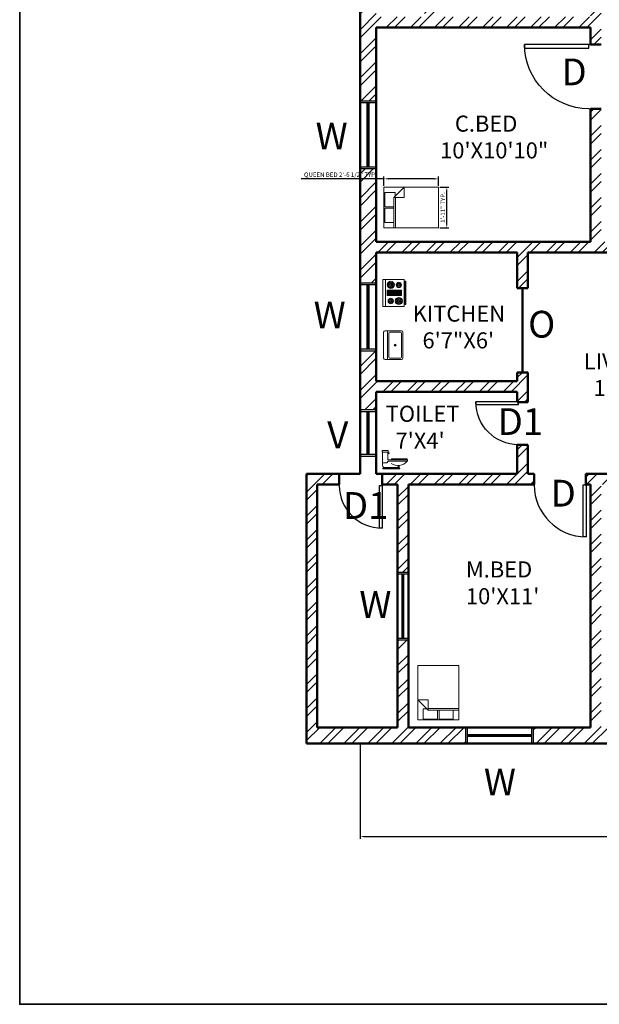
# Model space of a CAD drawing. Units: inches. Extents: x -31842 to -29388, y 18869 to 19743.
# Tile 1 of 12: x -31842 to -31517, y 18869 to 19420. Entities that reach past the tile are written whole.
import ezdxf

# ---------------------------------------------------------------- set-up
doc = ezdxf.new("R2010")
doc.units = ezdxf.units.IN
for name, color, linetype, lineweight in [('A-ANNO-DIMS', 2, 'Continuous', 18), ('A-ANNO-SYMB', 2, 'Continuous', 18), ('A-ANNO-TTLB', 7, 'Continuous', 35), ('A-AREA-IDEN', 3, 'Continuous', 18), ('A-DOOR', 3, 'Continuous', 25), ('A-FLOR-FIXT', 8, 'Continuous', 18), ('A-FURN', 8, 'Continuous', 18), ('A-GLAZ', 4, 'Continuous', 25), ('A-WALL', 7, 'Continuous', 50), ('A-WALL-PATT', 8, 'Continuous', 13)]:
    doc.layers.add(name, color=color, linetype=linetype, lineweight=lineweight)
doc.styles.get("Standard").update_dxf_attribs({"font": 'arial.ttf'})
doc.dimstyles.new('ISO-25', dxfattribs={"dimtxt": 2.5, "dimasz": 2.5, "dimexe": 1.25, "dimexo": 0.625, "dimtad": 1, "dimdec": 0, "dimlunit": 3, "dimtxsty": 'Standard', "dimcen": 2.5, "dimadec": 0, "dimazin": 0, "dimtfac": 1, "dimtdec": 0, "dimtmove": 0, "dimatfit": 3, "dimfxl": 1, "dimarcsym": 0})

# ---------------------------------------------------------------- blocks, each defined once
blk = doc.blocks.new('*U8')
for p, q in [((0, 0), (0, -100)), ((750, 0), (750, -100))]:
    blk.add_line(p, q)
blk.add_lwpolyline([(0, 0), (0, 750), (43.75, 750), (43.75, 0)], close=True)
blk.add_arc((0, 0), 750, 0, 90)
blk = doc.blocks.new('Bed - Queen')
for p, q in [((0, -80.00003), (0, 0)), ((0, 0), (59.99999, 0)), ((59.99999, 0), (59.99999, -80.00003)), ((0, -14.4), (44.8, -14.4)), ((7.99999, -1.2), (28.79998, -1.2)), ((7.99999, -14.4), (7.99999, -1.2)), ((28.79998, -1.2), (28.79998, -14.4)), ((31.19999, -1.2), (51.99999, -1.2)), ((31.19999, -14.4), (31.19999, -1.2)), ((59.99999, -29.6), (44.8, -14.4)), ((44.8, -14.4), (44.8, -29.6)), ((51.99999, -1.2), (51.99999, -16.4)), ((44.8, -16.8), (0, -16.8)), ((51.99999, -16.4), (46.79936, -16.4)), ((44.8, -29.6), (59.99999, -29.6)), ((59.99999, -80.00003), (0, -80.00003))]:
    blk.add_line(p, q)
blk = doc.blocks.new('Toilet - side')
for p, q in [((0.5, 5), (0.5, 22)), ((7.5, 22), (7.5, 12)), ((7.5, 21), (9, 21)), ((9, 20), (7.5, 20)), ((9, 21), (9, 20)), ((32.5, 13), (12, 13)), ((12, 13), (12, 12)), ((32.5, 12), (32.5, 13)), ((6, 8), (0.5, 8)), ((22, 2), (2, 2)), ((2, 2), (2, 1)), ((8, 10), (6, 8)), ((7.5, 12), (33, 12)), ((33, 10), (8, 10)), ((21, 4.5), (21, 2)), ((22, 2), (22, 4.5)), ((22, 1), (22, 2)), ((33, 12), (33, 10))]:
    blk.add_line(p, q)
for points in [[(0, 22), (0, 24), (8, 24), (8, 22)], [(1, 0), (1, 1), (23, 1), (23, 0)]]:
    blk.add_lwpolyline(points, close=True)
for centre, radius, start, end in [((3.8, 4.8), 3.26, 175.6013, 237.5288), ((20.3, 20.7), 16.2, 238.1872, 318.7702)]:
    blk.add_arc(centre, radius, start, end)
blk = doc.blocks.new('Range-Oven - 30 in top')
for p, q in [((0, -3), (30, -3)), ((12, -6), (18, -6)), ((13, -20), (13, -6)), ((14, -6), (14, -20)), ((15, -20), (15, -6)), ((16, -6), (16, -20)), ((17, -20), (17, -6)), ((18, -20), (12, -20)), ((6, -24), (6, -25)), ((8, -25), (8, -24)), ((22, -25), (22, -24)), ((24, -24), (24, -25))]:
    blk.add_line(p, q)
for points in [[(0, -24), (0, 0), (30, 0), (30, -24)], [(12, -21), (12, -5), (18, -5), (18, -21)], [(2, -26), (2, -25), (28, -25), (28, -26)]]:
    blk.add_lwpolyline(points, close=True)
for centre, radius in [((6, -9), 4), ((6, -9), 3), ((6, -9), 2), ((6, -9), 1), ((24, -9), 3), ((24, -9), 2), ((24, -9), 1), ((6, -18), 3), ((6, -18), 2), ((6, -18), 1), ((24, -18), 4), ((24, -18), 3), ((24, -18), 2), ((24, -18), 1)]:
    blk.add_circle(centre, radius)
blk = doc.blocks.new('Sink-single - 30 in top')
blk.add_line((-15, -3.999996), (15, -3.999996))
for points in [[(-13.5, 0), (13.5, 0)], [(-15, -18.499996), (-15, -1.5)], [(-13.5, -17.499996), (-13.5, -6.499996)], [(-12.5, -5.499996), (12.5, -5.499996)], [(13.5, -6.499996), (13.5, -17.499996)], [(15, -1.5), (15, -18.499996)], [(13.5, -19.999996), (-13.5, -19.999996)], [(12.5, -18.499996), (-12.5, -18.499996)]]:
    blk.add_lwpolyline(points)
for radius in [1, 0.5]:
    blk.add_circle((0, -11.999996), radius)
for centre, radius, start, end in [((-13.5, -1.5), 1.5, 90, 180), ((-12.5, -6.499996), 1, 90, 180), ((12.5, -6.499996), 1, 0, 90), ((13.5, -1.5), 1.5, 0, 90), ((-13.5, -18.499996), 1.5, 180, 270), ((-12.5, -17.499996), 1, 180, 270), ((12.5, -17.499996), 1, 270, 0), ((13.5, -18.499996), 1.5, 270, 0)]:
    blk.add_arc(centre, radius, start, end)
blk = doc.blocks.new('*D197')
at = {"layer": 'A-ANNO-DIMS', "color": 0, "lineweight": -2, "transparency": 16777216}
for p, q in [((-31651.45, 19014.34), (-31651.45, 18961.52)), ((-31119.45, 19014.34), (-31119.45, 18961.52)), ((-31648.95, 18962.77), (-31121.95, 18962.77))]:
    blk.add_line(p, q, dxfattribs=at)
at = {"layer": 'A-ANNO-DIMS', "color": 0, "transparency": 16777216}
for points in [[(-31648.95, 18963.19), (-31648.95, 18962.35), (-31651.45, 18962.77)], [(-31121.95, 18963.19), (-31121.95, 18962.35), (-31119.45, 18962.77)]]:
    blk.add_solid(points, dxfattribs=at)
at = {"layer": 'Defpoints', "color": 0, "transparency": 16777216}
for p in [(-31651.45, 19014.96), (-31119.45, 19014.96), (-31119.45, 18962.77)]:
    blk.add_point(p, dxfattribs=at)
at = {"layer": 'A-ANNO-DIMS', "color": 0, "transparency": 16777216, "insert": (-31385.45, 18971.4), "char_height": 2.5, "attachment_point": 5}
blk.add_mtext('{\\H6.4x;44\'-4"}', dxfattribs=at)
blk = doc.blocks.new('WIN-3FT')
for p, q in [((0, 36), (9, 36)), ((4, 0), (4, 36)), ((4.5, 0), (4.5, 36)), ((5, 0), (5, 36)), ((0, 0), (9, 0))]:
    blk.add_line(p, q)
blk = doc.blocks.new('WIN-3FT-B')
for p, q in [((0, 36), (6, 36)), ((2.5, 0), (2.5, 36)), ((3, 0), (3, 36)), ((3.5, 0), (3.5, 36)), ((0, 0), (6, 0))]:
    blk.add_line(p, q)
blk = doc.blocks.new('WIN-2FT')
for p, q in [((0, 24), (9, 24)), ((4, 0), (4, 24)), ((4.5, 0), (4.5, 24)), ((5, 0), (5, 24)), ((0, 0), (9, 0))]:
    blk.add_line(p, q)
blk = doc.blocks.new('*D219')
at = {"layer": 'A-ANNO-DIMS', "color": 0, "lineweight": -2, "transparency": 16777216}
for p, q in [((-31638.11, 19331.23), (-31684.46, 19331.23)), ((-31638.11, 19327.27), (-31638.11, 19332.48)), ((-31610.03, 19331.23), (-31635.61, 19331.23)), ((-31607.53, 19327.27), (-31607.53, 19332.48))]:
    blk.add_line(p, q, dxfattribs=at)
at = {"layer": 'A-ANNO-DIMS', "color": 0, "transparency": 16777216}
for points in [[(-31635.61, 19331.65), (-31635.61, 19330.82), (-31638.11, 19331.23)], [(-31610.03, 19331.65), (-31610.03, 19330.82), (-31607.53, 19331.23)]]:
    blk.add_solid(points, dxfattribs=at)
at = {"layer": 'Defpoints', "color": 0, "transparency": 16777216}
for p in [(-31638.11, 19331.23), (-31638.11, 19326.65), (-31607.53, 19326.65)]:
    blk.add_point(p, dxfattribs=at)
at = {"layer": 'A-ANNO-DIMS', "color": 0, "transparency": 16777216, "insert": (-31662.54, 19333.23), "char_height": 2.5, "attachment_point": 5}
blk.add_mtext('QUEEN BED 2\'-6 1/2" TYP.', dxfattribs=at)
blk = doc.blocks.new('*D220')
at = {"layer": 'A-ANNO-DIMS', "color": 0, "lineweight": -2, "transparency": 16777216}
for p, q in [((-31606.91, 19326.65), (-31601.69, 19326.65)), ((-31602.94, 19306.21), (-31602.94, 19324.15)), ((-31606.91, 19303.71), (-31601.69, 19303.71))]:
    blk.add_line(p, q, dxfattribs=at)
at = {"layer": 'A-ANNO-DIMS', "color": 0, "transparency": 16777216}
for points in [[(-31603.36, 19324.15), (-31602.53, 19324.15), (-31602.94, 19326.65)], [(-31603.36, 19306.21), (-31602.53, 19306.21), (-31602.94, 19303.71)]]:
    blk.add_solid(points, dxfattribs=at)
at = {"layer": 'Defpoints', "color": 0, "transparency": 16777216}
for p in [(-31607.53, 19326.65), (-31602.94, 19326.65), (-31607.53, 19303.71)]:
    blk.add_point(p, dxfattribs=at)
at = {"layer": 'A-ANNO-DIMS', "color": 0, "transparency": 16777216, "insert": (-31604.82, 19315.18), "char_height": 2.5, "attachment_point": 5, "rotation": 90}
blk.add_mtext('1\'-11" TYP.', dxfattribs=at)

msp = doc.modelspace()

# ---------------------------------------------------------------- hatches: boundary and pattern name
at = {"layer": 'A-WALL-PATT'}
h = msp.add_hatch(dxfattribs=at)
h.set_pattern_fill('ANSI32', color=256)
h.paths.add_polyline_path([(-31119.45, 19656.96), (-31254.45, 19656.96), (-31254.45, 19614.96), (-31277.45, 19614.96), (-31277.45, 19605.96), (-31254.45, 19605.96), (-31254.45, 19555.2), (-31248.45, 19555.2), (-31248.45, 19605.96), (-31240.75, 19605.96), (-31240.75, 19614.96), (-31248.45, 19614.96), (-31248.45, 19650.96), (-31128.45, 19650.96), (-31128.45, 19614.96), (-31216.75, 19614.96), (-31216.75, 19605.96), (-31128.45, 19605.96), (-31128.45, 19559.96), (-31119.45, 19559.96)])
h.paths.add_polyline_path([(-31153.94, 19473.06), (-31153.92, 19475.96), (-31248.45, 19475.96), (-31248.45, 19519.2), (-31251.45, 19519.2), (-31254.45, 19519.2), (-31254.45, 19497.96), (-31267.62, 19497.96), (-31267.62, 19491.96), (-31254.45, 19491.96), (-31254.45, 19465.12), (-31248.45, 19465.12), (-31248.45, 19469.96), (-31161.45, 19469.96), (-31161.45, 19458.96), (-31155.45, 19458.96), (-31155.45, 19469.96), (-31153.94, 19469.96)])
h.paths.add_polyline_path([(-31119.45, 19521.96), (-31128.45, 19521.96), (-31128.45, 19475.96), (-31129.92, 19475.96), (-31129.92, 19469.96), (-31128.45, 19469.96), (-31128.45, 19421.96), (-31155.45, 19421.96), (-31155.45, 19432.96), (-31161.45, 19432.96), (-31161.45, 19421.96), (-31248.45, 19421.96), (-31248.45, 19441.12), (-31254.45, 19441.12), (-31254.45, 19406.17), (-31248.45, 19406.17), (-31248.45, 19415.96), (-31128.45, 19415.96), (-31128.45, 19375.96), (-31119.45, 19375.96)])
h.paths.add_polyline_path([(-31315.45, 19614.96), (-31366.45, 19614.96), (-31366.45, 19605.96), (-31344.45, 19605.96), (-31344.45, 19456.39), (-31338.45, 19456.39), (-31338.45, 19491.96), (-31328.43, 19491.96), (-31328.43, 19497.96), (-31338.45, 19497.96), (-31338.45, 19605.96), (-31315.45, 19605.96)])
h.paths.add_polyline_path([(-31404.45, 19614.96), (-31455.1, 19614.96), (-31455.1, 19605.96), (-31432.45, 19605.96), (-31432.45, 19497.96), (-31448.67, 19497.96), (-31448.67, 19491.96), (-31432.45, 19491.96), (-31432.45, 19456.39), (-31429.07, 19456.39), (-31426.45, 19456.39), (-31426.45, 19605.96), (-31404.45, 19605.96)])
h.paths.add_polyline_path([(-31493.1, 19614.96), (-31516.45, 19614.96), (-31516.45, 19656.96), (-31651.45, 19656.96), (-31651.45, 19559.96), (-31642.45, 19559.96), (-31642.45, 19605.96), (-31556.65, 19605.96), (-31556.65, 19614.96), (-31642.45, 19614.96), (-31642.45, 19650.96), (-31522.45, 19650.96), (-31522.45, 19614.96), (-31532.65, 19614.96), (-31532.65, 19613.66), (-31532.65, 19610.46), (-31532.65, 19605.96), (-31522.45, 19605.96), (-31522.45, 19541.95), (-31516.45, 19541.95), (-31516.45, 19605.96), (-31493.1, 19605.96)])
h.paths.add_polyline_path([(-31642.45, 19521.96), (-31651.45, 19521.96), (-31651.45, 19374.96), (-31642.45, 19374.96), (-31642.45, 19415.96), (-31522.45, 19415.96), (-31522.45, 19406.54), (-31516.45, 19406.54), (-31516.45, 19441.56), (-31522.45, 19441.56), (-31522.45, 19421.96), (-31609.45, 19421.96), (-31609.45, 19432.96), (-31615.45, 19432.96), (-31615.45, 19421.96), (-31642.45, 19421.96), (-31642.45, 19469.96), (-31641.6, 19469.96), (-31641.6, 19475.96), (-31642.45, 19475.96)])
h.paths.add_polyline_path([(-31516.45, 19491.96), (-31506.54, 19491.96), (-31506.54, 19497.96), (-31516.45, 19497.96), (-31516.45, 19505.95), (-31522.45, 19505.95), (-31522.45, 19475.96), (-31617.6, 19475.96), (-31617.6, 19469.96), (-31615.45, 19469.96), (-31615.45, 19458.96), (-31609.45, 19458.96), (-31609.45, 19469.96), (-31522.45, 19469.96), (-31522.45, 19465.56), (-31516.45, 19465.56)])
h.paths.add_polyline_path([(-31248.45, 19370.17), (-31251.45, 19370.17), (-31254.45, 19370.17), (-31254.45, 19297.96), (-31338.45, 19297.96), (-31338.45, 19420.39), (-31344.45, 19420.39), (-31344.45, 19413.96), (-31346.02, 19413.96), (-31346.02, 19407.96), (-31344.45, 19407.96), (-31344.45, 19291.96), (-31213.45, 19291.96), (-31213.45, 19275.43), (-31207.45, 19275.43), (-31207.45, 19291.96), (-31128.45, 19291.96), (-31128.45, 19274.96), (-31119.45, 19274.96), (-31119.45, 19337.96), (-31128.45, 19337.96), (-31128.45, 19297.96), (-31248.45, 19297.96)])
h.paths.add_polyline_path([(-31426.45, 19407.96), (-31424.99, 19407.96), (-31424.99, 19410.83), (-31424.95, 19413.96), (-31426.45, 19413.96), (-31426.45, 19420.39), (-31432.45, 19420.39), (-31432.45, 19295.96), (-31516.45, 19295.96), (-31516.45, 19370.54), (-31522.45, 19370.54), (-31522.45, 19295.96), (-31642.45, 19295.96), (-31642.45, 19336.96), (-31651.45, 19336.96), (-31651.45, 19272.96), (-31642.45, 19272.96), (-31642.45, 19289.96), (-31563.45, 19289.96), (-31563.45, 19270.05), (-31557.45, 19270.05), (-31557.45, 19289.96), (-31426.45, 19289.96)])
h.paths.add_polyline_path([(-31557.45, 19222.83), (-31563.45, 19222.83), (-31563.45, 19217.96), (-31642.45, 19217.96), (-31642.45, 19234.96), (-31651.45, 19234.96), (-31651.45, 19201.96), (-31642.45, 19201.96), (-31642.45, 19211.96), (-31563.45, 19211.96), (-31563.45, 19206.27), (-31562.72, 19206.27), (-31559.53, 19206.27), (-31557.45, 19206.18)])
h.paths.add_polyline_path([(-31553.97, 19163.65), (-31553.95, 19165.96), (-31557.45, 19165.96), (-31557.45, 19182.18), (-31563.45, 19182.18), (-31563.45, 19165.96), (-31639.16, 19165.96), (-31639.16, 19159.96), (-31630.45, 19159.96), (-31630.45, 19110.96), (-31624.45, 19110.96), (-31624.45, 19159.96), (-31553.97, 19159.96)])
h.paths.add_polyline_path([(-31663.16, 19165.96), (-31681.45, 19165.96), (-31681.45, 19014.96), (-31592.45, 19014.96), (-31592.45, 19023.96), (-31624.45, 19023.96), (-31624.45, 19072.96), (-31630.45, 19072.96), (-31630.45, 19023.96), (-31675.45, 19023.96), (-31675.45, 19159.96), (-31663.16, 19159.96)])
h.paths.add_polyline_path([(-31516.45, 19159.96), (-31505.99, 19159.96), (-31505.99, 19165.96), (-31524.95, 19165.96), (-31524.95, 19159.96), (-31522.45, 19159.96), (-31522.45, 19023.96), (-31554.45, 19023.96), (-31554.45, 19014.96), (-31471.45, 19014.96), (-31471.45, 19023.96), (-31516.45, 19023.96)])
h.paths.add_polyline_path([(-31337.45, 19023.96), (-31382.45, 19023.96), (-31382.45, 19159.96), (-31299.75, 19159.96), (-31299.75, 19165.96), (-31344.45, 19165.96), (-31382.45, 19165.96), (-31382.45, 19407.96), (-31382.02, 19413.96), (-31388.95, 19413.96), (-31388.95, 19407.96), (-31388.45, 19407.96), (-31388.45, 19165.96), (-31432.45, 19165.96), (-31469.99, 19165.96), (-31469.99, 19159.96), (-31432.45, 19159.96), (-31388.45, 19159.96), (-31388.45, 19023.96), (-31433.45, 19023.96), (-31433.45, 19014.96), (-31337.45, 19014.96)])
h.paths.add_polyline_path([(-31216.45, 19023.96), (-31248.45, 19023.96), (-31248.45, 19159.96), (-31245.93, 19159.96), (-31245.93, 19162.87), (-31245.93, 19165.96), (-31254.45, 19165.96), (-31263.75, 19165.96), (-31263.75, 19159.96), (-31254.45, 19159.96), (-31254.45, 19023.96), (-31299.45, 19023.96), (-31299.45, 19014.96), (-31216.45, 19014.96)])
h.paths.add_polyline_path([(-31089.45, 19165.96), (-31110.75, 19165.96), (-31110.75, 19159.96), (-31095.45, 19159.96), (-31095.45, 19023.96), (-31140.45, 19023.96), (-31140.45, 19072.96), (-31146.45, 19072.96), (-31146.45, 19023.96), (-31178.45, 19023.96), (-31178.45, 19014.96), (-31089.45, 19014.96)])
h.paths.add_polyline_path([(-31134.75, 19165.96), (-31207.45, 19165.96), (-31207.45, 19182.5), (-31213.45, 19182.5), (-31213.45, 19165.96), (-31216.93, 19165.96), (-31216.93, 19159.96), (-31146.45, 19159.96), (-31146.45, 19110.96), (-31140.45, 19110.96), (-31140.45, 19159.96), (-31134.75, 19159.96)])
h.paths.add_polyline_path([(-31119.45, 19236.96), (-31128.45, 19236.96), (-31128.45, 19219.96), (-31207.45, 19219.96), (-31207.45, 19227.12), (-31213.45, 19227.12), (-31213.45, 19206.5), (-31207.45, 19206.5), (-31207.45, 19213.96), (-31128.45, 19213.96), (-31128.45, 19202.96), (-31119.45, 19202.96)])

# ---------------------------------------------------------------- linework, layer by layer
at = {"layer": 'A-ANNO-TTLB'}
msp.add_lwpolyline([(-31842.18, 19743.36), (-29387.67, 19743.36), (-29387.67, 18868.82), (-31842.18, 18868.82)], close=True, dxfattribs=at)
at = {"layer": 'A-GLAZ'}
for p, q in [((-31651.45, 19374.96), (-31642.45, 19374.96)), ((-31651.45, 19336.96), (-31642.45, 19336.96)), ((-31651.45, 19272.96), (-31642.45, 19272.96)), ((-31651.45, 19234.96), (-31642.45, 19234.96)), ((-31651.45, 19201.96), (-31642.45, 19201.96)), ((-31651.45, 19175.96), (-31642.45, 19175.96)), ((-31630.45, 19110.96), (-31624.45, 19110.96)), ((-31630.45, 19072.96), (-31624.45, 19072.96)), ((-31592.45, 19023.96), (-31592.45, 19014.96)), ((-31554.45, 19023.96), (-31554.45, 19014.96))]:
    msp.add_line(p, q, dxfattribs=at)
at = {"layer": 'A-WALL'}
for p, q in [((-31651.45, 19165.96), (-31651.45, 19656.96)), ((-31642.45, 19415.96), (-31522.45, 19415.96)), ((-31642.45, 19295.96), (-31642.45, 19415.96)), ((-31522.45, 19406.54), (-31522.45, 19415.96)), ((-31522.45, 19406.54), (-31516.45, 19406.54)), ((-31522.45, 19295.96), (-31522.45, 19370.54)), ((-31522.45, 19370.54), (-31516.45, 19370.54)), ((-31642.45, 19295.96), (-31522.45, 19295.96)), ((-31642.45, 19289.96), (-31563.45, 19289.96)), ((-31642.45, 19217.96), (-31642.45, 19289.96)), ((-31563.45, 19270.05), (-31563.45, 19289.96)), ((-31557.45, 19289.96), (-31426.45, 19289.96)), ((-31557.45, 19270.05), (-31557.45, 19289.96)), ((-31563.45, 19270.05), (-31557.45, 19270.05)), ((-31560.45, 19222.83), (-31560.45, 19270.05)), ((-31563.45, 19217.96), (-31563.45, 19222.83)), ((-31563.45, 19222.83), (-31557.45, 19222.83)), ((-31557.45, 19206.18), (-31557.45, 19222.83)), ((-31642.45, 19217.96), (-31563.45, 19217.96)), ((-31642.45, 19165.96), (-31642.45, 19211.96)), ((-31642.45, 19211.96), (-31563.45, 19211.96)), ((-31563.45, 19206.18), (-31563.45, 19211.96)), ((-31563.45, 19206.18), (-31557.45, 19206.18)), ((-31563.45, 19165.96), (-31563.45, 19182.18)), ((-31563.45, 19182.18), (-31557.45, 19182.18)), ((-31557.45, 19165.96), (-31557.45, 19182.18)), ((-31681.45, 19165.96), (-31651.45, 19165.96)), ((-31681.45, 19014.96), (-31681.45, 19165.96)), ((-31663.16, 19165.96), (-31663.16, 19159.96)), ((-31642.45, 19165.96), (-31563.45, 19165.96)), ((-31639.16, 19165.96), (-31639.16, 19159.96)), ((-31557.45, 19165.96), (-31553.95, 19165.96)), ((-31553.95, 19159.96), (-31553.95, 19165.96)), ((-31524.95, 19159.96), (-31524.95, 19165.96)), ((-31524.95, 19165.96), (-31505.99, 19165.96)), ((-31675.45, 19159.96), (-31663.16, 19159.96)), ((-31675.45, 19023.96), (-31675.45, 19159.96)), ((-31639.16, 19159.96), (-31630.45, 19159.96)), ((-31630.45, 19023.96), (-31630.45, 19159.96)), ((-31624.45, 19023.96), (-31624.45, 19159.96)), ((-31624.45, 19159.96), (-31553.95, 19159.96)), ((-31524.95, 19159.96), (-31522.45, 19159.96)), ((-31522.45, 19023.96), (-31522.45, 19159.96)), ((-31630.45, 19023.96), (-31675.45, 19023.96)), ((-31522.45, 19023.96), (-31624.45, 19023.96)), ((-31089.45, 19014.96), (-31681.45, 19014.96))]:
    msp.add_line(p, q, dxfattribs=at)

# ---------------------------------------------------------------- block references
at = {"layer": 'A-DOOR'}
for p, xscale, yscale, zscale, rotation in [((-31523.33, 19406.54), -0.0480027575407148, 0.0480027575407148, 0.0480027575407148, 90), ((-31562.72, 19206.27), -0.0319267259435146, 0.0319267259435146, 0.0319267259435146, 90), ((-31639.17, 19159.53), 0.0320000000000009, 0.0320000000000009, 0.0320000000000009, 180), ((-31524.93, 19159.78), 0.0387159446673275, 0.0387159446673275, 0.0387159446673275, 180)]:
    msp.add_blockref('*U8', p, dxfattribs=dict(at, xscale=xscale, yscale=yscale, zscale=zscale, rotation=rotation))
at = {"layer": 'A-FLOR-FIXT', "rotation": 90}
for name, p, xscale, yscale, zscale in [('Range-Oven - 30 in top', (-31638.82, 19274.83), -0.501109879279097, 0.501109879279097, 0.501109879279097), ('Sink-single - 30 in top', (-31638.29, 19238.07), -0.537483841617589, 0.537483841617589, 0.537483841617589)]:
    msp.add_blockref(name, p, dxfattribs=dict(at, xscale=xscale, yscale=yscale, zscale=zscale))
at = {"layer": 'A-FLOR-FIXT', "xscale": 0.4314503559530352, "yscale": 0.4314503559530352, "zscale": 0.4314503559530352}
msp.add_blockref('Toilet - side', (-31639.14, 19168.7), dxfattribs=at)
at = {"layer": 'A-FURN', "xscale": 0.382279819255463, "yscale": 0.382279819255463, "zscale": 0.382279819255463}
for p, rotation in [((-31638.11, 19303.71), 90), ((-31596.21, 19028.1), 180)]:
    msp.add_blockref('Bed - Queen', p, dxfattribs=dict(at, rotation=rotation))
at = {"layer": 'A-GLAZ'}
for name, p in [('WIN-3FT', (-31651.45, 19337.96)), ('WIN-3FT', (-31651.45, 19235.96)), ('WIN-2FT', (-31651.45, 19176.96)), ('WIN-3FT-B', (-31630.45, 19073.96))]:
    msp.add_blockref(name, p, dxfattribs=at)
at = {"layer": 'A-GLAZ', "rotation": 269.9999999999837}
msp.add_blockref('WIN-3FT', (-31591.45, 19023.96), dxfattribs=at)

# ---------------------------------------------------------------- texts
at = {"layer": 'A-ANNO-SYMB', "char_height": 15, "attachment_point": 1}
for s, insert in [('{D}', (-31538.64, 19398.64)), ('{W}', (-31676.41, 19362.71)), ('{W}', (-31677.51, 19262.51)), ('{O}', (-31557.36, 19257.29)), ('{D1}', (-31574.39, 19202.77)), ('{V}', (-31669.89, 19195.31)), ('{D}', (-31544.72, 19162.63)), ('{D1}', (-31661.08, 19155.76)), ('{W}', (-31651.91, 19100.3)), ('{W}', (-31582.15, 19000.88))]:
    msp.add_mtext_dynamic_manual_height_columns(s, width=533.5224, gutter_width=12.5, heights=[0], dxfattribs=dict(at, insert=insert))
at = {"layer": 'A-AREA-IDEN', "char_height": 2.5, "attachment_point": 1}
for s, insert in [('{\\H3.6x;   C.BED\\P10\'X10\'10"}', (-31606.65, 19366.67)), ('{\\H3.6x;  KITCHEN\\P    6\'7"X6\'}', (-31627.54, 19260.25)), ('{\\H3.6x;LIVING/DINING\\P  16\'10"X11\'1"}', (-31526.21, 19233.53)), ("{\\H3.6x; TOILET\\P   7'X4'}", (-31639.89, 19204.14)), ("{\\H3.6x;   M.BED\\P   10'X11'}", (-31600.46, 19116.93))]:
    msp.add_mtext_dynamic_manual_height_columns(s, width=652.6959, gutter_width=12.5, heights=[0], dxfattribs=dict(at, insert=insert))

# ---------------------------------------------------------------- dimensions: what is measured, and where the dimension line sits
at = {"layer": 'A-ANNO-DIMS'}
for base, p1, p2, angle, text, picture, middle in [((-31638.11, 19331.23), (-31607.53, 19326.65), (-31638.11, 19326.65), 180, 'QUEEN BED <> TYP.', '*D219', (-31662.54, 19333.23)), ((-31602.94, 19326.65), (-31607.53, 19303.71), (-31607.53, 19326.65), 90, '<> TYP.', '*D220', (-31604.82, 19315.18))]:
    dim = msp.add_linear_dim(base=base, p1=p1, p2=p2, angle=angle, text=text, dimstyle='ISO-25', override={"dimdec": 1, "dimlfac": 1, "dimrnd": 0, "dimzin": 1, "dimdsep": 46, "dimlunit": 4, "dimfrac": 2}, dxfattribs=at)
    dim.commit()
    dim.dimension.update_dxf_attribs({"geometry": picture, "text_midpoint": middle})
dim = msp.add_linear_dim(base=(-31119.45, 18962.77), p1=(-31651.45, 19014.96), p2=(-31119.45, 19014.96), text='{\\H6.4x;<>}', dimstyle='ISO-25', override={"dimclrd": 0, "dimclre": 0, "dimclrt": 0}, dxfattribs=at)
dim.commit()
dim.dimension.update_dxf_attribs({"geometry": '*D197', "text_midpoint": (-31385.45, 18971.4)})

doc.saveas('drawing.dxf')
